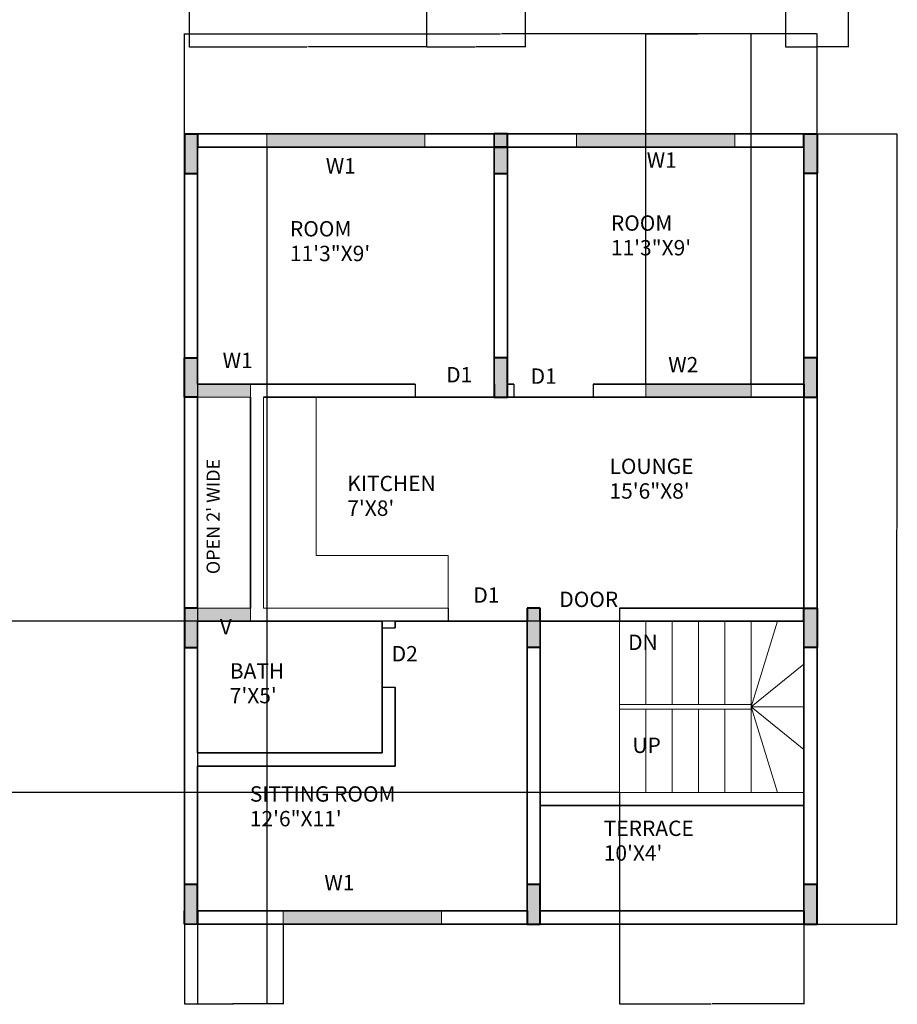
# Model space of a CAD drawing. Units: millimetres. Extents: x 1831 to 2754, y 1517 to 2450.
# Tile 2 of 4: x 2355 to 2754, y 1517 to 1965. Entities that reach past the tile are written whole.
import ezdxf

# ---------------------------------------------------------------- set-up
doc = ezdxf.new("R2010")
doc.units = ezdxf.units.MM
for name, color, linetype, lineweight in [('A-ANNO-DIMS', 2, 'Continuous', 18), ('A-ANNO-TEXT', 7, 'Continuous', 18), ('A-AREA-IDEN', 7, 'Continuous', 18), ('A-COLS', 7, 'Continuous', 40), ('A-DETL-REFP', 8, 'Continuous', 13), ('A-DOOR', 3, 'Continuous', 25), ('A-FLOR-CASE', 8, 'Continuous', 18), ('A-FLOR-STRS', 7, 'Continuous', 18), ('A-GLAZ', 4, 'Continuous', 18), ('A-WALL', 7, 'Continuous', 35)]:
    doc.layers.add(name, color=color, linetype=linetype, lineweight=lineweight)
doc.layers.add('A-COLS-PATT', color=18, linetype='Continuous', lineweight=13, true_color=0x000000)
doc.layers.add('A-GLAZ-PATT', color=252, linetype='Continuous', lineweight=13, true_color=0x939598)
doc.styles.get("Standard").update_dxf_attribs({"font": 'arial.ttf'})
doc.dimstyles.get("Standard").update_dxf_attribs({"dimtxt": 0.18, "dimasz": 0.18, "dimexe": 0.18, "dimexo": 0.0625, "dimgap": 0.09, "dimtad": 0, "dimtih": 1, "dimtoh": 1, "dimdec": 4, "dimzin": 0, "dimdsep": 46, "dimtxsty": 'Standard', "dimcen": 0.09, "dimadec": 0, "dimazin": 0, "dimtfac": 1, "dimtdec": 4, "dimtofl": 0, "dimtmove": 0, "dimatfit": 3, "dimfxl": 1, "dimtolj": 1, "dimtzin": 0, "dimarcsym": 0})

# ---------------------------------------------------------------- blocks, each defined once
blk = doc.blocks.new('*D38')
at = {"layer": 'A-ANNO-DIMS', "color": 0, "lineweight": -2, "transparency": 16777216}
for p, q in [((2429.6, 1913.28), (2429.6, 1958.89)), ((2429.78, 1958.71), (2573.31, 1958.71)), ((2717.42, 1958.71), (2573.89, 1958.71)), ((2717.6, 1913.28), (2717.6, 1958.89))]:
    blk.add_line(p, q, dxfattribs=at)
at = {"layer": 'A-ANNO-DIMS', "color": 0, "transparency": 16777216}
for points in [[(2429.78, 1958.74), (2429.78, 1958.68), (2429.6, 1958.71)], [(2717.42, 1958.74), (2717.42, 1958.68), (2717.6, 1958.71)]]:
    blk.add_solid(points, dxfattribs=at)
at = {"layer": 'Defpoints', "color": 0, "transparency": 16777216}
for p in [(2717.6, 1958.71), (2429.6, 1913.22), (2717.6, 1913.22)]:
    blk.add_point(p, dxfattribs=at)
at = {"layer": 'A-ANNO-DIMS', "color": 0, "transparency": 16777216, "insert": (2573.6, 1958.71), "char_height": 0.18, "attachment_point": 5}
blk.add_mtext('\\A1;288', dxfattribs=at)
blk = doc.blocks.new('*D39')
at = {"layer": 'A-ANNO-DIMS', "color": 0, "lineweight": -2, "transparency": 16777216}
for p, q in [((2717.66, 1913.22), (2754.11, 1913.22)), ((2753.93, 1913.04), (2753.93, 1733.4)), ((2753.93, 1553.4), (2753.93, 1733.03)), ((2717.66, 1553.22), (2754.11, 1553.22))]:
    blk.add_line(p, q, dxfattribs=at)
at = {"layer": 'A-ANNO-DIMS', "color": 0, "transparency": 16777216}
for points in [[(2753.9, 1913.04), (2753.96, 1913.04), (2753.93, 1913.22)], [(2753.9, 1553.4), (2753.96, 1553.4), (2753.93, 1553.22)]]:
    blk.add_solid(points, dxfattribs=at)
at = {"layer": 'Defpoints', "color": 0, "transparency": 16777216}
for p in [(2717.6, 1913.22), (2753.93, 1913.22), (2717.6, 1553.22)]:
    blk.add_point(p, dxfattribs=at)
at = {"layer": 'A-ANNO-DIMS', "color": 0, "transparency": 16777216, "insert": (2753.93, 1733.22), "char_height": 0.18, "attachment_point": 5}
blk.add_mtext('\\A1;360', dxfattribs=at)
blk = doc.blocks.new('*D40')
at = {"layer": 'A-ANNO-DIMS', "color": 0, "lineweight": -2, "transparency": 16777216}
for p, q in [((2429.6, 1553.15), (2429.6, 1516.71)), ((2474.6, 1553.15), (2474.6, 1516.71)), ((2429.78, 1516.89), (2451.88, 1516.89)), ((2474.42, 1516.89), (2452.33, 1516.89))]:
    blk.add_line(p, q, dxfattribs=at)
at = {"layer": 'A-ANNO-DIMS', "color": 0, "transparency": 16777216}
for points in [[(2429.78, 1516.92), (2429.78, 1516.86), (2429.6, 1516.89)], [(2474.42, 1516.92), (2474.42, 1516.86), (2474.6, 1516.89)]]:
    blk.add_solid(points, dxfattribs=at)
at = {"layer": 'Defpoints', "color": 0, "transparency": 16777216}
for p in [(2429.6, 1553.22), (2474.6, 1553.22), (2474.6, 1516.89)]:
    blk.add_point(p, dxfattribs=at)
at = {"layer": 'A-ANNO-DIMS', "color": 0, "transparency": 16777216, "insert": (2452.1, 1516.89), "char_height": 0.18, "attachment_point": 5}
blk.add_mtext('\\A1;45', dxfattribs=at)
blk = doc.blocks.new('*D41')
at = {"layer": 'A-ANNO-DIMS', "color": 0, "lineweight": -2, "transparency": 16777216}
for p, q in [((2435.6, 1907.15), (2435.6, 1516.71)), ((2467.1, 1907.15), (2467.1, 1516.71)), ((2435.78, 1516.89), (2451.03, 1516.89)), ((2466.92, 1516.89), (2451.68, 1516.89))]:
    blk.add_line(p, q, dxfattribs=at)
at = {"layer": 'A-ANNO-DIMS', "color": 0, "transparency": 16777216}
for points in [[(2435.78, 1516.92), (2435.78, 1516.86), (2435.6, 1516.89)], [(2466.92, 1516.92), (2466.92, 1516.86), (2467.1, 1516.89)]]:
    blk.add_solid(points, dxfattribs=at)
at = {"layer": 'Defpoints', "color": 0, "transparency": 16777216}
for p in [(2435.6, 1907.22), (2467.1, 1907.22), (2467.1, 1516.89)]:
    blk.add_point(p, dxfattribs=at)
at = {"layer": 'A-ANNO-DIMS', "color": 0, "transparency": 16777216, "insert": (2451.35, 1516.89), "char_height": 0.18, "attachment_point": 5}
blk.add_mtext('\\A1;31.5', dxfattribs=at)
blk = doc.blocks.new('*D42')
at = {"layer": 'A-ANNO-DIMS', "color": 0, "lineweight": -2, "transparency": 16777216}
for p, q in [((2639.6, 1799.28), (2639.6, 1958.89)), ((2639.78, 1958.71), (2663.38, 1958.71)), ((2687.42, 1958.71), (2663.82, 1958.71)), ((2687.6, 1799.28), (2687.6, 1958.89))]:
    blk.add_line(p, q, dxfattribs=at)
at = {"layer": 'A-ANNO-DIMS', "color": 0, "transparency": 16777216}
for points in [[(2639.78, 1958.74), (2639.78, 1958.68), (2639.6, 1958.71)], [(2687.42, 1958.74), (2687.42, 1958.68), (2687.6, 1958.71)]]:
    blk.add_solid(points, dxfattribs=at)
at = {"layer": 'Defpoints', "color": 0, "transparency": 16777216}
for p in [(2687.6, 1958.71), (2639.6, 1799.22), (2687.6, 1799.22)]:
    blk.add_point(p, dxfattribs=at)
at = {"layer": 'A-ANNO-DIMS', "color": 0, "transparency": 16777216, "insert": (2663.6, 1958.71), "char_height": 0.18, "attachment_point": 5}
blk.add_mtext('\\A1;48', dxfattribs=at)
blk = doc.blocks.new('*D43')
at = {"layer": 'A-ANNO-DIMS', "color": 0, "lineweight": -2, "transparency": 16777216}
for p, q in [((2627.6, 1613.15), (2627.6, 1516.71)), ((2711.6, 1613.15), (2711.6, 1516.71)), ((2627.78, 1516.89), (2669.38, 1516.89)), ((2711.42, 1516.89), (2669.82, 1516.89))]:
    blk.add_line(p, q, dxfattribs=at)
at = {"layer": 'A-ANNO-DIMS', "color": 0, "transparency": 16777216}
for points in [[(2627.78, 1516.92), (2627.78, 1516.86), (2627.6, 1516.89)], [(2711.42, 1516.92), (2711.42, 1516.86), (2711.6, 1516.89)]]:
    blk.add_solid(points, dxfattribs=at)
at = {"layer": 'Defpoints', "color": 0, "transparency": 16777216}
for p in [(2627.6, 1613.22), (2711.6, 1613.22), (2711.6, 1516.89)]:
    blk.add_point(p, dxfattribs=at)
at = {"layer": 'A-ANNO-DIMS', "color": 0, "transparency": 16777216, "insert": (2669.6, 1516.89), "char_height": 0.18, "attachment_point": 5}
blk.add_mtext('\\A1;84', dxfattribs=at)
blk = doc.blocks.new('*D44')
at = {"layer": 'A-ANNO-DIMS', "color": 0, "lineweight": -2, "transparency": 16777216}
for p, q in [((2627.54, 1691.22), (1955.06, 1691.22)), ((1955.24, 1691.04), (1955.24, 1652.4)), ((1955.24, 1613.4), (1955.24, 1652.03)), ((2627.54, 1613.22), (1955.06, 1613.22))]:
    blk.add_line(p, q, dxfattribs=at)
at = {"layer": 'A-ANNO-DIMS', "color": 0, "transparency": 16777216}
for points in [[(1955.21, 1691.04), (1955.27, 1691.04), (1955.24, 1691.22)], [(1955.21, 1613.4), (1955.27, 1613.4), (1955.24, 1613.22)]]:
    blk.add_solid(points, dxfattribs=at)
at = {"layer": 'Defpoints', "color": 0, "transparency": 16777216}
for p in [(1955.24, 1691.22), (2627.6, 1691.22), (2627.6, 1613.22)]:
    blk.add_point(p, dxfattribs=at)
at = {"layer": 'A-ANNO-DIMS', "color": 0, "transparency": 16777216, "insert": (1955.24, 1652.22), "char_height": 0.18, "attachment_point": 5}
blk.add_mtext('\\A1;78', dxfattribs=at)
blk = doc.blocks.new('*D67')
at = {"layer": 'A-ANNO-DIMS', "color": 0, "lineweight": -2, "transparency": 16777216}
for p, q in [((2431.76, 2019.5), (2431.76, 1952.75)), ((2539.76, 2019.5), (2539.76, 1952.75)), ((2431.94, 1952.93), (2485.48, 1952.93)), ((2539.58, 1952.93), (2486.04, 1952.93))]:
    blk.add_line(p, q, dxfattribs=at)
at = {"layer": 'A-ANNO-DIMS', "color": 0, "transparency": 16777216}
for points in [[(2431.94, 1952.96), (2431.94, 1952.9), (2431.76, 1952.93)], [(2539.58, 1952.96), (2539.58, 1952.9), (2539.76, 1952.93)]]:
    blk.add_solid(points, dxfattribs=at)
at = {"layer": 'Defpoints', "color": 0, "transparency": 16777216}
for p in [(2431.76, 2019.57), (2539.76, 2019.57), (2539.76, 1952.93)]:
    blk.add_point(p, dxfattribs=at)
at = {"layer": 'A-ANNO-DIMS', "color": 0, "transparency": 16777216, "insert": (2485.76, 1952.93), "char_height": 0.18, "attachment_point": 5}
blk.add_mtext('\\A1;108', dxfattribs=at)
blk = doc.blocks.new('*D68')
at = {"layer": 'A-ANNO-DIMS', "color": 0, "lineweight": -2, "transparency": 16777216}
for p, q in [((2539.76, 2019.5), (2539.76, 1952.75)), ((2584.76, 2019.5), (2584.76, 1952.75)), ((2539.94, 1952.93), (2562.04, 1952.93)), ((2584.58, 1952.93), (2562.48, 1952.93))]:
    blk.add_line(p, q, dxfattribs=at)
at = {"layer": 'A-ANNO-DIMS', "color": 0, "transparency": 16777216}
for points in [[(2539.94, 1952.96), (2539.94, 1952.9), (2539.76, 1952.93)], [(2584.58, 1952.96), (2584.58, 1952.9), (2584.76, 1952.93)]]:
    blk.add_solid(points, dxfattribs=at)
at = {"layer": 'Defpoints', "color": 0, "transparency": 16777216}
for p in [(2539.76, 2019.57), (2584.76, 2019.57), (2584.76, 1952.93)]:
    blk.add_point(p, dxfattribs=at)
at = {"layer": 'A-ANNO-DIMS', "color": 0, "transparency": 16777216, "insert": (2562.26, 1952.93), "char_height": 0.18, "attachment_point": 5}
blk.add_mtext('\\A1;45', dxfattribs=at)
blk = doc.blocks.new('*D69')
at = {"layer": 'A-ANNO-DIMS', "color": 0, "lineweight": -2, "transparency": 16777216}
for p, q in [((2703.26, 2055.5), (2703.26, 1952.75)), ((2731.76, 2019.5), (2731.76, 1952.75)), ((2703.44, 1952.93), (2717.18, 1952.93)), ((2731.58, 1952.93), (2717.83, 1952.93))]:
    blk.add_line(p, q, dxfattribs=at)
at = {"layer": 'A-ANNO-DIMS', "color": 0, "transparency": 16777216}
for points in [[(2703.44, 1952.96), (2703.44, 1952.9), (2703.26, 1952.93)], [(2731.58, 1952.96), (2731.58, 1952.9), (2731.76, 1952.93)]]:
    blk.add_solid(points, dxfattribs=at)
at = {"layer": 'Defpoints', "color": 0, "transparency": 16777216}
for p in [(2703.26, 2055.57), (2731.76, 2019.57), (2731.76, 1952.93)]:
    blk.add_point(p, dxfattribs=at)
at = {"layer": 'A-ANNO-DIMS', "color": 0, "transparency": 16777216, "insert": (2717.51, 1952.93), "char_height": 0.18, "attachment_point": 5}
blk.add_mtext('\\A1;28.5', dxfattribs=at)

msp = doc.modelspace()

# ---------------------------------------------------------------- hatches: boundary and pattern name
at = {"layer": 'A-COLS-PATT'}
h = msp.add_hatch(color=256, dxfattribs=at)
h.dxf.hatch_style = 1
h.paths.add_polyline_path([(1997.569, 1916.378), (1997.569, 1922.378), (1991.569, 1922.378), (1991.569, 1904.378), (1997.569, 1904.378)])
h.paths.add_polyline_path([(1997.569, 1820.378), (1991.569, 1820.378), (1991.569, 1802.378), (1997.569, 1802.378), (1997.569, 1808.378)])
h.paths.add_polyline_path([(2138.569, 1820.378), (2132.569, 1820.378), (2132.569, 1802.378), (2138.569, 1802.378), (2138.569, 1808.378)])
h.paths.add_polyline_path([(2138.569, 1916.378), (2138.569, 1922.378), (2132.569, 1922.378), (2132.569, 1904.378), (2138.569, 1904.378)])
h.paths.add_polyline_path([(2279.569, 1922.378), (2273.569, 1922.378), (2273.569, 1904.378), (2279.569, 1904.378)])
h.paths.add_polyline_path([(2279.569, 1820.378), (2273.569, 1820.378), (2273.569, 1808.378), (2273.569, 1802.378), (2279.569, 1802.378)])
h.paths.add_polyline_path([(1997.569, 1706.378), (1991.569, 1706.378), (1991.569, 1688.378), (1997.569, 1688.378), (1997.569, 1700.378)])
h.paths.add_polyline_path([(2153.569, 1700.378), (2153.569, 1706.378), (2147.569, 1706.378), (2147.569, 1688.378), (2153.569, 1688.378)])
h.paths.add_polyline_path([(2279.569, 1706.378), (2273.569, 1706.378), (2273.569, 1700.378), (2273.569, 1688.378), (2279.569, 1688.378)])
h.paths.add_polyline_path([(2435.602, 1907.216), (2435.602, 1913.216), (2429.602, 1913.216), (2429.602, 1895.216), (2435.602, 1895.216)])
h.paths.add_polyline_path([(2435.602, 1811.216), (2429.602, 1811.216), (2429.602, 1793.216), (2435.602, 1793.216), (2435.602, 1799.216)])
h.paths.add_polyline_path([(2576.602, 1811.216), (2570.602, 1811.216), (2570.602, 1799.216), (2570.602, 1793.216), (2576.602, 1793.216)])
h.paths.add_polyline_path([(2576.602, 1907.216), (2570.602, 1907.216), (2570.602, 1895.216), (2576.602, 1895.216)])
h.paths.add_polyline_path([(2576.602, 1913.216), (2570.602, 1913.216), (2570.602, 1907.216), (2576.602, 1907.216)])
h.paths.add_polyline_path([(2717.602, 1811.216), (2711.602, 1811.216), (2711.602, 1799.216), (2711.602, 1793.216), (2717.602, 1793.216)])
h.paths.add_polyline_path([(2435.602, 1691.216), (2435.602, 1697.216), (2429.602, 1697.216), (2429.602, 1679.216), (2435.602, 1679.216)])
h.paths.add_polyline_path([(2591.602, 1691.216), (2591.602, 1697.216), (2585.602, 1697.216), (2585.602, 1691.216), (2585.602, 1679.216), (2591.602, 1679.216)])
h.paths.add_polyline_path([(2717.602, 1697.216), (2711.602, 1697.216), (2711.602, 1691.216), (2711.602, 1679.216), (2717.602, 1679.216)])
h.paths.add_polyline_path([(2717.602, 1913.216), (2711.602, 1913.216), (2711.602, 1907.216), (2711.602, 1895.216), (2717.602, 1895.216)])
h.paths.add_polyline_path([(1997.569, 1580.378), (1991.569, 1580.378), (1991.569, 1568.378), (1997.569, 1568.378)])
h.paths.add_polyline_path([(1997.569, 1568.378), (1991.569, 1568.378), (1991.569, 1562.378), (1997.569, 1562.378)])
h.paths.add_polyline_path([(2153.569, 1580.378), (2147.569, 1580.378), (2147.569, 1568.378), (2147.569, 1562.378), (2153.569, 1562.378)])
h.paths.add_polyline_path([(2279.569, 1580.378), (2273.569, 1580.378), (2273.569, 1568.378), (2273.569, 1562.378), (2279.569, 1562.378)])
h.paths.add_polyline_path([(2435.602, 1571.216), (2429.602, 1571.216), (2429.602, 1553.216), (2435.602, 1553.216)])
h.paths.add_polyline_path([(2717.602, 1571.216), (2711.602, 1571.216), (2711.602, 1559.216), (2711.602, 1553.216), (2717.602, 1553.216)])
h.paths.add_polyline_path([(2591.602, 1571.216), (2585.602, 1571.216), (2585.602, 1559.216), (2585.602, 1553.216), (2591.602, 1553.216)])
at = {"layer": 'A-GLAZ-PATT'}
h = msp.add_hatch(color=256, dxfattribs=at)
h.dxf.hatch_style = 1
h.paths.add_polyline_path([(2539.102, 1913.216), (2503.102, 1913.216), (2467.102, 1913.216), (2467.102, 1907.216), (2539.102, 1907.216)])
h.paths.add_polyline_path([(2680.102, 1913.216), (2608.102, 1913.216), (2608.102, 1907.216), (2644.102, 1907.216), (2680.102, 1907.216)])
h.paths.add_polyline_path([(2687.602, 1799.216), (2663.602, 1799.216), (2639.602, 1799.216), (2639.602, 1793.216), (2687.602, 1793.216)])
h.paths.add_polyline_path([(2459.602, 1799.216), (2435.602, 1799.216), (2435.602, 1793.216), (2459.602, 1793.216)])
h.paths.add_polyline_path([(2459.602, 1697.216), (2435.602, 1697.216), (2435.602, 1691.216), (2459.602, 1691.216)])
h.paths.add_polyline_path([(2546.602, 1559.216), (2510.602, 1559.216), (2474.602, 1559.216), (2474.602, 1553.216), (2546.602, 1553.216)])

# ---------------------------------------------------------------- linework, layer by layer
at = {"layer": 'A-COLS'}
for p, q in [((2429.602, 1913.216), (2435.602, 1913.216)), ((2429.602, 1913.216), (2429.602, 1895.216)), ((2435.602, 1913.216), (2435.602, 1907.216)), ((2576.602, 1913.216), (2570.602, 1913.216)), ((2576.602, 1907.216), (2576.602, 1913.216)), ((2711.602, 1907.216), (2711.602, 1913.216)), ((2711.602, 1913.216), (2717.602, 1913.216)), ((2717.602, 1913.216), (2717.602, 1895.216)), ((2570.602, 1907.216), (2576.602, 1907.216)), ((2576.602, 1907.216), (2570.602, 1907.216)), ((2429.602, 1895.216), (2435.602, 1895.216)), ((2570.602, 1895.216), (2576.602, 1895.216)), ((2717.602, 1895.216), (2711.602, 1895.216)), ((2429.602, 1793.216), (2429.602, 1811.216)), ((2429.602, 1811.216), (2435.602, 1811.216)), ((2576.602, 1811.216), (2570.602, 1811.216)), ((2576.602, 1793.216), (2576.602, 1811.216)), ((2717.602, 1811.216), (2711.602, 1811.216)), ((2717.602, 1793.216), (2717.602, 1811.216)), ((2570.602, 1799.216), (2570.602, 1793.216)), ((2570.602, 1799.216), (2570.602, 1799.216)), ((2711.602, 1799.216), (2711.602, 1793.216)), ((2435.602, 1793.216), (2429.602, 1793.216)), ((2570.602, 1793.216), (2576.602, 1793.216)), ((2711.602, 1793.216), (2717.602, 1793.216)), ((2435.602, 1697.216), (2429.602, 1697.216)), ((2429.602, 1697.216), (2429.602, 1679.216)), ((2591.602, 1697.216), (2585.602, 1697.216)), ((2585.602, 1697.216), (2585.602, 1691.216)), ((2591.602, 1697.216), (2585.602, 1697.216)), ((2591.602, 1691.216), (2591.602, 1697.216)), ((2711.602, 1691.216), (2711.602, 1697.216)), ((2711.602, 1697.216), (2717.602, 1697.216)), ((2717.602, 1697.216), (2717.602, 1679.216)), ((2429.602, 1679.216), (2435.602, 1679.216)), ((2591.602, 1679.216), (2585.602, 1679.216)), ((2717.602, 1679.216), (2711.602, 1679.216)), ((2435.602, 1571.216), (2429.602, 1571.216)), ((2435.602, 1553.216), (2435.602, 1571.216)), ((2591.602, 1571.216), (2585.602, 1571.216)), ((2591.602, 1553.216), (2591.602, 1571.216)), ((2717.602, 1571.216), (2711.602, 1571.216)), ((2717.602, 1553.216), (2717.602, 1571.216)), ((2429.602, 1553.216), (2429.602, 1559.216)), ((2435.602, 1559.216), (2435.602, 1553.216)), ((2585.602, 1559.216), (2585.602, 1553.216)), ((2711.602, 1559.216), (2711.602, 1553.216)), ((2585.602, 1553.216), (2591.602, 1553.216)), ((2711.602, 1553.216), (2717.602, 1553.216))]:
    msp.add_line(p, q, dxfattribs=at)
at = {"layer": 'A-DETL-REFP'}
for p in [(2637.202, 1691.216), (2646.802, 1691.216), (2656.402, 1691.216), (2666.002, 1691.216)]:
    msp.add_point(p, dxfattribs=at)
at = {"layer": 'A-DOOR'}
for p, q in [((2534.602, 1799.216), (2534.602, 1793.216)), ((2579.602, 1799.216), (2579.602, 1793.216)), ((2615.602, 1799.216), (2615.602, 1793.216)), ((2534.602, 1793.216), (2570.602, 1793.216)), ((2579.602, 1793.216), (2579.602, 1793.216)), ((2549.602, 1697.216), (2549.602, 1691.216)), ((2627.602, 1697.216), (2627.602, 1691.216)), ((2519.602, 1688.216), (2525.602, 1688.216)), ((2519.602, 1688.216), (2519.602, 1661.216)), ((2519.602, 1661.216), (2525.602, 1661.216))]:
    msp.add_line(p, q, dxfattribs=at)
at = {"layer": 'A-FLOR-CASE'}
for p, q in [((2465.602, 1793.216), (2465.602, 1697.216)), ((2465.602, 1793.216), (2465.602, 1769.216)), ((2489.602, 1769.216), (2489.602, 1793.216)), ((2489.602, 1769.216), (2489.602, 1721.216)), ((2489.602, 1721.216), (2549.602, 1721.216)), ((2549.602, 1697.216), (2549.602, 1721.216)), ((2465.602, 1697.216), (2549.602, 1697.216)), ((2549.602, 1697.216), (2465.602, 1697.216))]:
    msp.add_line(p, q, dxfattribs=at)
at = {"layer": 'A-FLOR-STRS'}
for p, q in [((2627.602, 1691.216), (2627.602, 1607.216)), ((2627.602, 1691.216), (2675.602, 1691.216)), ((2627.602, 1691.216), (2687.602, 1691.216)), ((2639.602, 1653.216), (2639.602, 1691.216)), ((2663.602, 1691.216), (2651.602, 1691.216)), ((2651.602, 1691.216), (2651.602, 1653.216)), ((2663.602, 1653.216), (2663.602, 1691.216)), ((2711.602, 1691.216), (2675.602, 1691.216)), ((2675.602, 1691.216), (2687.602, 1691.216)), ((2687.602, 1691.216), (2675.602, 1691.216)), ((2675.602, 1691.216), (2675.602, 1653.216)), ((2687.602, 1691.216), (2687.602, 1613.216)), ((2687.602, 1691.216), (2711.602, 1691.216)), ((2687.602, 1652.216), (2699.602, 1691.216)), ((2699.602, 1691.216), (2687.602, 1652.216)), ((2711.602, 1691.216), (2711.602, 1613.216)), ((2711.602, 1691.216), (2711.602, 1652.216)), ((2687.602, 1652.216), (2711.602, 1671.716)), ((2687.602, 1653.216), (2627.602, 1653.216)), ((2687.602, 1651.216), (2627.602, 1651.216)), ((2639.602, 1613.216), (2639.602, 1651.216)), ((2651.602, 1651.216), (2651.602, 1613.216)), ((2663.602, 1613.216), (2663.602, 1651.216)), ((2675.602, 1651.216), (2675.602, 1613.216)), ((2687.602, 1652.216), (2711.602, 1652.216)), ((2687.602, 1652.216), (2699.602, 1613.216)), ((2699.602, 1613.216), (2687.602, 1652.216)), ((2687.602, 1652.216), (2711.602, 1632.716)), ((2711.602, 1613.216), (2711.602, 1652.216)), ((2711.602, 1613.216), (2711.602, 1652.216)), ((2711.602, 1613.216), (2627.602, 1613.216)), ((2651.602, 1613.216), (2639.602, 1613.216)), ((2675.602, 1613.216), (2663.602, 1613.216)), ((2687.602, 1613.216), (2711.602, 1613.216))]:
    msp.add_line(p, q, dxfattribs=at)
at = {"layer": 'A-GLAZ'}
for p, q in [((2503.102, 1913.216), (2467.102, 1913.216)), ((2467.102, 1913.216), (2467.102, 1907.216)), ((2539.102, 1907.216), (2539.102, 1913.216)), ((2608.102, 1907.216), (2608.102, 1913.216)), ((2608.102, 1913.216), (2680.102, 1913.216)), ((2680.102, 1913.216), (2680.102, 1907.216)), ((2467.102, 1907.216), (2539.102, 1907.216)), ((2644.102, 1907.216), (2608.102, 1907.216)), ((2435.602, 1799.216), (2435.602, 1793.216)), ((2459.602, 1793.216), (2459.602, 1799.216)), ((2663.602, 1799.216), (2639.602, 1799.216)), ((2639.602, 1799.216), (2639.602, 1793.216)), ((2687.602, 1793.216), (2687.602, 1799.216)), ((2435.602, 1793.216), (2459.602, 1793.216)), ((2639.602, 1793.216), (2687.602, 1793.216)), ((2459.602, 1697.216), (2435.602, 1697.216)), ((2435.602, 1691.216), (2435.602, 1697.216)), ((2459.602, 1697.216), (2459.602, 1691.216)), ((2510.602, 1559.216), (2474.602, 1559.216)), ((2474.602, 1559.216), (2474.602, 1553.216)), ((2546.602, 1553.216), (2546.602, 1559.216)), ((2474.602, 1553.216), (2546.602, 1553.216))]:
    msp.add_line(p, q, dxfattribs=at)
at = {"layer": 'A-WALL'}
for p, q in [((2429.602, 1913.216), (2717.602, 1913.216)), ((2429.602, 1553.216), (2429.602, 1913.216)), ((2429.602, 1913.216), (2717.602, 1913.216)), ((2435.602, 1913.216), (2570.602, 1913.216)), ((2570.602, 1913.216), (2503.102, 1913.216)), ((2570.602, 1913.216), (2570.602, 1895.216)), ((2717.602, 1913.216), (2717.602, 1553.216)), ((2435.602, 1907.216), (2570.602, 1907.216)), ((2435.602, 1799.216), (2435.602, 1907.216)), ((2435.602, 1907.216), (2570.602, 1907.216)), ((2570.602, 1907.216), (2570.602, 1799.216)), ((2576.602, 1907.216), (2711.602, 1907.216)), ((2576.602, 1799.216), (2576.602, 1907.216)), ((2576.602, 1907.216), (2711.602, 1907.216)), ((2711.602, 1907.216), (2644.102, 1907.216)), ((2711.602, 1907.216), (2711.602, 1799.216)), ((2534.602, 1799.216), (2435.602, 1799.216)), ((2576.602, 1799.216), (2579.602, 1799.216)), ((2579.602, 1799.216), (2576.602, 1799.216)), ((2711.602, 1799.216), (2615.602, 1799.216)), ((2615.602, 1799.216), (2711.602, 1799.216)), ((2711.602, 1799.216), (2663.602, 1799.216)), ((2435.602, 1697.216), (2435.602, 1793.216)), ((2459.602, 1793.216), (2459.602, 1697.216)), ((2459.602, 1697.216), (2459.602, 1793.216)), ((2465.602, 1793.216), (2711.602, 1793.216)), ((2711.602, 1793.216), (2711.602, 1697.216)), ((2711.602, 1697.216), (2627.602, 1697.216)), ((2435.602, 1691.216), (2435.602, 1631.216)), ((2519.602, 1691.216), (2435.602, 1691.216)), ((2519.602, 1631.216), (2519.602, 1691.216)), ((2519.602, 1691.216), (2519.602, 1688.216)), ((2585.602, 1691.216), (2525.602, 1691.216)), ((2525.602, 1691.216), (2525.602, 1688.216)), ((2585.602, 1559.216), (2585.602, 1691.216)), ((2591.602, 1691.216), (2591.602, 1559.216)), ((2591.602, 1691.216), (2711.602, 1691.216)), ((2711.602, 1691.216), (2711.602, 1607.216)), ((2525.602, 1661.216), (2525.602, 1631.216)), ((2435.602, 1631.216), (2519.602, 1631.216)), ((2525.602, 1631.216), (2525.602, 1625.216)), ((2441.602, 1625.216), (2435.602, 1625.216)), ((2435.602, 1625.216), (2435.602, 1559.216)), ((2525.602, 1625.216), (2441.602, 1625.216)), ((2591.602, 1613.216), (2591.602, 1613.216)), ((2711.602, 1607.216), (2711.602, 1613.216)), ((2711.602, 1607.216), (2591.602, 1607.216)), ((2711.602, 1559.216), (2711.602, 1607.216)), ((2435.602, 1559.216), (2585.602, 1559.216)), ((2435.602, 1559.216), (2585.602, 1559.216)), ((2585.602, 1559.216), (2510.602, 1559.216)), ((2591.602, 1559.216), (2711.602, 1559.216)), ((2717.602, 1553.216), (2429.602, 1553.216))]:
    msp.add_line(p, q, dxfattribs=at)

# ---------------------------------------------------------------- texts
at = {"layer": 'A-ANNO-TEXT'}
for s, p in [('W1', (2493.941, 1895.163)), ('W1', (2640.06, 1897.77)), ('W1', (2446.973, 1806.519)), ('W2', (2649.845, 1804.564)), ('D1', (2548.735, 1800.002)), ('D1', (2587.222, 1799.35)), ('D1', (2561.13, 1699.625)), ('DOOR', (2600.269, 1697.67)), ('V', (2445.669, 1685.286)), ('DN', (2631.58, 1678.116)), ('D2', (2523.947, 1672.902)), ('UP', (2633.537, 1631.187)), ('W1', (2493.288, 1568.615))]:
    msp.add_text(s, height=7, dxfattribs=at).set_placement(p)
msp.add_text("OPEN 2' WIDE", height=6, rotation=90, dxfattribs=at).set_placement((2445.669, 1712.661))
at = {"layer": 'A-AREA-IDEN'}
for s, p in [('ROOM', (2623.752, 1869.091)), ('ROOM', (2477.633, 1866.484)), ('11\'3"X9\'', (2477.633, 1855.239)), ('11\'3"X9\'', (2623.752, 1857.847)), ('LOUNGE', (2623.1, 1758.287)), ('KITCHEN', (2503.725, 1750.465)), ('15\'6"X8\'', (2623.1, 1747.042)), ("7'X8'", (2503.725, 1739.22)), ('BATH', (2450.235, 1665.08)), ("7'X5'", (2450.235, 1653.836)), ('SITTING ROOM', (2459.368, 1609.026)), ('12\'6"X11\'', (2459.368, 1597.781)), ('TERRACE', (2620.491, 1593.383)), ("10'X4'", (2620.491, 1582.138))]:
    msp.add_text(s, height=7, dxfattribs=at).set_placement(p)

# ---------------------------------------------------------------- dimensions: what is measured, and where the dimension line sits
at = {"layer": 'A-ANNO-DIMS'}
for base, p1, p2, override, picture, middle in [((2731.758, 1952.933), (2703.258, 2055.566), (2731.758, 2019.566), {"dimdec": 1, "dimlfac": 1, "dimrnd": 0, "dimzin": 0, "dimdsep": 46, "dimlunit": 2}, '*D69', (2717.508, 1952.933)), ((2539.758, 1952.933), (2431.758, 2019.566), (2539.758, 2019.566), {"dimdec": 0, "dimlfac": 1, "dimrnd": 0, "dimzin": 0, "dimdsep": 46, "dimlunit": 2}, '*D67', (2485.758, 1952.933)), ((2584.758, 1952.933), (2539.758, 2019.566), (2584.758, 2019.566), {"dimdec": 0, "dimlfac": 1, "dimrnd": 0, "dimzin": 0, "dimdsep": 46, "dimlunit": 2}, '*D68', (2562.258, 1952.933)), ((2717.602, 1958.708), (2429.602, 1913.216), (2717.602, 1913.216), {"dimdec": 0, "dimlfac": 1, "dimrnd": 0, "dimzin": 0, "dimdsep": 46, "dimlunit": 2}, '*D38', (2573.602, 1958.708)), ((2687.602, 1958.708), (2639.602, 1799.216), (2687.602, 1799.216), {"dimdec": 0, "dimlfac": 1, "dimrnd": 0, "dimzin": 0, "dimdsep": 46, "dimlunit": 2}, '*D42', (2663.602, 1958.708)), ((2467.102, 1516.886), (2435.602, 1907.216), (2467.102, 1907.216), {"dimdec": 1, "dimlfac": 1, "dimrnd": 0, "dimzin": 0, "dimdsep": 46, "dimlunit": 2}, '*D41', (2451.352, 1516.886)), ((2711.602, 1516.886), (2627.602, 1613.216), (2711.602, 1613.216), {"dimdec": 0, "dimlfac": 1, "dimrnd": 0, "dimzin": 0, "dimdsep": 46, "dimlunit": 2}, '*D43', (2669.602, 1516.886)), ((2474.602, 1516.886), (2429.602, 1553.216), (2474.602, 1553.216), {"dimdec": 0, "dimlfac": 1, "dimrnd": 0, "dimzin": 0, "dimdsep": 46, "dimlunit": 2}, '*D40', (2452.102, 1516.886))]:
    dim = msp.add_linear_dim(base=base, p1=p1, p2=p2, dimstyle='Standard', override=override, dxfattribs=at)
    dim.commit()
    dim.dimension.update_dxf_attribs({"geometry": picture, "text_midpoint": middle})
for base, p1, p2, picture, middle in [((2753.932, 1913.216), (2717.602, 1553.216), (2717.602, 1913.216), '*D39', (2753.932, 1733.216)), ((1955.239, 1691.216), (2627.602, 1613.216), (2627.602, 1691.216), '*D44', (1955.239, 1652.216))]:
    dim = msp.add_linear_dim(base=base, p1=p1, p2=p2, angle=90, dimstyle='Standard', override={"dimdec": 0, "dimlfac": 1, "dimrnd": 0, "dimzin": 0, "dimdsep": 46, "dimlunit": 2}, dxfattribs=at)
    dim.commit()
    dim.dimension.update_dxf_attribs({"geometry": picture, "text_midpoint": middle})

doc.saveas('drawing.dxf')
